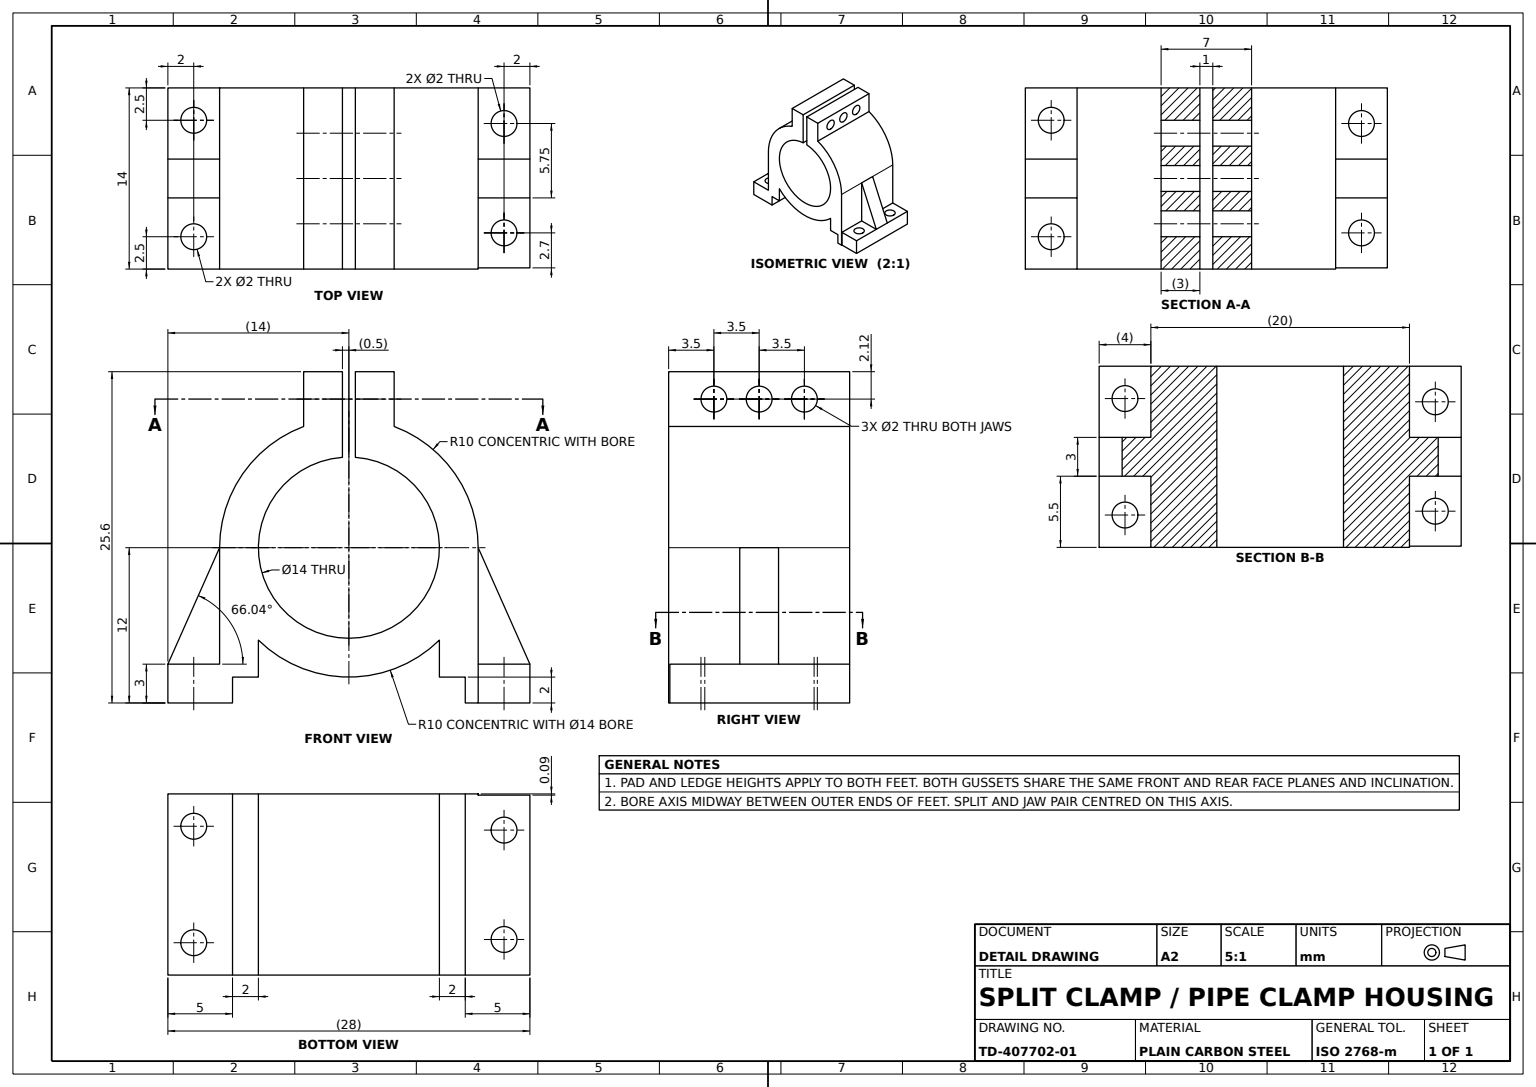
from build123d import *

# Parameters (mm, degrees)
BASE_BLOCK_SKETCH_R              = 10
BASE_BLOCK_SKETCH_R_2            = 7
BASE_BLOCK_DEPTH                 = 14
CLAMP_START                      = -14
CLAMP_RING_DEPTH                 = 14
SIDE_RIB_SKETCH_W                = 3.6
SIDE_RIB_SKETCH_H                = 14
SIDE_RIB_DEPTH                   = 3.5
RIB_START                        = -14
RIB_INFILL_DEPTH                 = 14
MOUNTING_EAR_A_SKETCH_W          = 4
MOUNTING_EAR_A_SKETCH_H          = 13.906308923
MOUNTING_EAR_A_DEPTH             = 3
MOUNTING_EAR_B_SKETCH_W          = 4
MOUNTING_EAR_B_SKETCH_H          = 14
MOUNTING_EAR_B_DEPTH             = 3
CLAMP_SLIT_A_SKETCH_W            = 2
CLAMP_SLIT_A_SKETCH_H            = 2
CLAMP_SLIT_A_DEPTH               = 56
CLAMP_SLIT_B_SKETCH_W            = 2
CLAMP_SLIT_B_SKETCH_H            = 2
CLAMP_SLIT_B_DEPTH               = 92
TRIANGULAR_RELIEF_CUT_DEPTH      = 54
TRIANGULAR_RELIEF_CUT_DEPTH_BACK = 33
TRIANGULAR_RELIEF_SKETCH_R       = 1
RIB_GROOVE_SKETCH_W              = 0.5
RIB_GROOVE_SKETCH_H              = 14
RIB_GROOVE_CUT_DEPTH             = 14
EAR_A_GUSSET_DEPTH               = 1.5
EAR_A_HOLES_SKETCH_R             = 1
EAR_A_HOLES_2X_2_DEPTH           = 6.5
EAR_B_GUSSET_DEPTH               = 1.5
EAR_B_HOLES_SKETCH_R             = 1
EAR_B_HOLES_2X_2_DEPTH           = 10


with BuildPart() as part:
    # Base Block Sketch → Base Block (new body)
    with BuildSketch(Plane(origin=(0, 0, 0), x_dir=(1, 0, 0), z_dir=(0, 1, 0))):
        with Locations(Location((0, 0, 0), (0, 0, 270))):
            Circle(BASE_BLOCK_SKETCH_R)
        with Locations(Location((0, 0, 0), (0, 0, 270))):
            Circle(BASE_BLOCK_SKETCH_R_2, mode=Mode.SUBTRACT)
    extrude(amount=BASE_BLOCK_DEPTH)

    # Clamp Ring Sketch → Clamp Ring (add)
    with BuildSketch(Plane(origin=(0, 14, 0), x_dir=(1, 0, 0), z_dir=(0, 1, 0)).offset(CLAMP_START)):
        with BuildLine():
            Line((-7, -12), (-7, -7.141428429))
            ThreePointArc((-7, -7.141428429), (-9.219544457, -3.872983346), (-10, 0))
            Line((-10, 0), (-10, -12))
            Line((-10, -12), (-7, -12))
        make_face()
        with BuildLine():
            Line((10, -12), (10, 0))
            ThreePointArc((10, 0), (9.219544457, -3.872983346), (7, -7.141428429))
            Line((7, -7.141428429), (7, -12))
            Line((7, -12), (10, -12))
        make_face()
    extrude(amount=CLAMP_RING_DEPTH)



with BuildPart() as body_2:
    # Side Rib Sketch → Side Rib (new, symmetric)
    with BuildSketch(Plane(origin=(0, 0, 0), x_dir=(0, 0, -1), z_dir=(1, 0, 0))):
        with Locations((11.8, 7)):
            Rectangle(SIDE_RIB_SKETCH_W, SIDE_RIB_SKETCH_H)
    extrude(amount=SIDE_RIB_DEPTH, both=True)


with BuildPart() as part_1:
    add(part.part)

    add(body_2.part)  # Rib Infill merges body 2
    # Rib Infill Sketch → Rib Infill (add)
    with BuildSketch(Plane(origin=(0, 14, 0), x_dir=(1, 0, 0), z_dir=(0, 1, 0)).offset(RIB_START)):
        with BuildLine():
            Line((0, 10), (-3.5, 10))
            Line((-3.5, 10), (-3.5, 9.367496998))
            ThreePointArc((-3.5, 9.367496998), (-1.778346145, 9.840603893), (0, 10))
        make_face()
        with BuildLine():
            Line((3.5, 10), (0, 10))
            ThreePointArc((0, 10), (1.778346145, 9.840603893), (3.5, 9.367496998))
            Line((3.5, 9.367496998), (3.5, 10))
        make_face()
    extrude(amount=RIB_INFILL_DEPTH)

    # Mounting Ear A Sketch → Mounting Ear A (add)
    with BuildSketch(Plane.XY.offset(12)):
        with Locations((12, 6.953154462)):
            Rectangle(MOUNTING_EAR_A_SKETCH_W, MOUNTING_EAR_A_SKETCH_H)
    extrude(amount=-MOUNTING_EAR_A_DEPTH)

    # Mounting Ear B Sketch → Mounting Ear B (add)
    with BuildSketch(Plane.XY.offset(12)):
        with Locations((-12, 7)):
            Rectangle(MOUNTING_EAR_B_SKETCH_W, MOUNTING_EAR_B_SKETCH_H)
    extrude(amount=-MOUNTING_EAR_B_DEPTH)

    # Clamp Slit A Sketch → Clamp Slit A (cut)
    with BuildSketch(Plane(origin=(0, 14, 0), x_dir=(1, 0, 0), z_dir=(0, 1, 0))):
        with Locations((-8, -11)):
            Rectangle(CLAMP_SLIT_A_SKETCH_W, CLAMP_SLIT_A_SKETCH_H)
    extrude(amount=-CLAMP_SLIT_A_DEPTH, mode=Mode.SUBTRACT)

    # Clamp Slit B Sketch → Clamp Slit B (cut)
    with BuildSketch(Plane(origin=(0, 14, 0), x_dir=(1, 0, 0), z_dir=(0, 1, 0))):
        with Locations((8, -11)):
            Rectangle(CLAMP_SLIT_B_SKETCH_W, CLAMP_SLIT_B_SKETCH_H)
    extrude(amount=-CLAMP_SLIT_B_DEPTH, mode=Mode.SUBTRACT)

    # Triangular Relief Sketch → Triangular Relief Cut (cut, two sides: drawn at the far end of the back side and taken through both)
    with BuildSketch(Plane(origin=(3.5, 0, 0), x_dir=(0, 0, -1), z_dir=(1, 0, 0)).offset(-TRIANGULAR_RELIEF_CUT_DEPTH_BACK)):
        with Locations((11.483748499, 7)):
            Circle(TRIANGULAR_RELIEF_SKETCH_R)
        with Locations((11.483748499, 3.5)):
            Circle(TRIANGULAR_RELIEF_SKETCH_R)
        with Locations((11.483748499, 10.5)):
            Circle(TRIANGULAR_RELIEF_SKETCH_R)
    extrude(amount=TRIANGULAR_RELIEF_CUT_DEPTH + TRIANGULAR_RELIEF_CUT_DEPTH_BACK, mode=Mode.SUBTRACT)

    # Rib Groove Sketch → Rib Groove Cut (cut)
    with BuildSketch(Plane(origin=(0, 0, -13.6), x_dir=(-1, 0, 0), z_dir=(0, 0, -1))):
        with Locations((0.25, 7)):
            Rectangle(RIB_GROOVE_SKETCH_W, RIB_GROOVE_SKETCH_H)
        with Locations((-0.25, 7)):
            Rectangle(RIB_GROOVE_SKETCH_W, RIB_GROOVE_SKETCH_H)
    extrude(amount=-RIB_GROOVE_CUT_DEPTH, mode=Mode.SUBTRACT)

    # Ear A Gusset Sketch → Ear A Gusset (add, symmetric)
    with BuildSketch(Plane(origin=(0, 7, 0), x_dir=(1, 0, 0), z_dir=(0, 1, 0))):
        Polygon((14, -9), (10, 0), (10, -9), align=None)
    extrude(amount=EAR_A_GUSSET_DEPTH, both=True)

    # Ear A Holes Sketch → Ear A Holes 2xØ2 (cut, symmetric)
    with BuildSketch(Plane(origin=(0, 0, 9), x_dir=(-1, 0, 0), z_dir=(0, 0, -1))):
        with Locations((-12, 11.203154462)):
            Circle(EAR_A_HOLES_SKETCH_R)
        with Locations((-12, 2.75)):
            Circle(EAR_A_HOLES_SKETCH_R)
    extrude(amount=EAR_A_HOLES_2X_2_DEPTH, both=True, mode=Mode.SUBTRACT)

    # Ear B Gusset Sketch → Ear B Gusset (add, symmetric)
    with BuildSketch(Plane(origin=(0, 7, 0), x_dir=(1, 0, 0), z_dir=(0, 1, 0))):
        Polygon((-10, 0), (-14, -9), (-10, -9), align=None)
    extrude(amount=EAR_B_GUSSET_DEPTH, both=True)

    # Ear B Holes Sketch → Ear B Holes 2xØ2 (cut, symmetric)
    with BuildSketch(Plane(origin=(0, 0, 9), x_dir=(-1, 0, 0), z_dir=(0, 0, -1))):
        with Locations((12, 2.5)):
            Circle(EAR_B_HOLES_SKETCH_R)
        with Locations((12, 11.5)):
            Circle(EAR_B_HOLES_SKETCH_R)
    extrude(amount=EAR_B_HOLES_2X_2_DEPTH, both=True, mode=Mode.SUBTRACT)


solid = part_1.part
